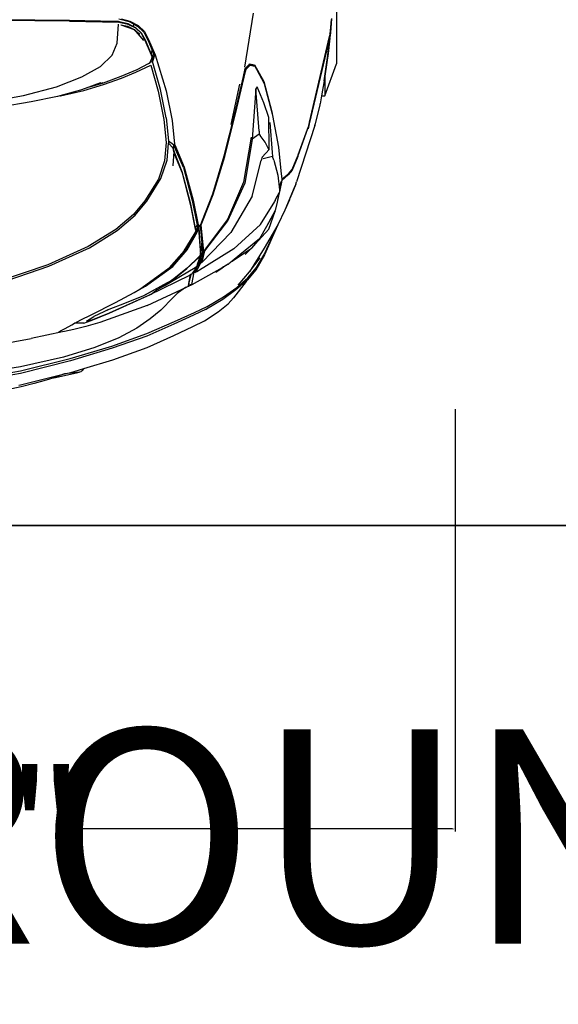
# Model space of a CAD drawing. Units: inches. Extents: x -4737294 to -4736756, y 1716389 to 1717040.
# Tile 5 of 25: x -4737133 to -4737096, y 1716424 to 1716491. Entities that reach past the tile are written whole.
import ezdxf

# ---------------------------------------------------------------- set-up
doc = ezdxf.new("R2010")
doc.units = ezdxf.units.IN
doc.header["$MEASUREMENT"] = 0
for name, color, linetype, lineweight in [('A-ANNO-DIMS', 2, 'Continuous', 18), ('A-ANNO-TEXT', 250, 'Continuous', 30), ('A-EQPM-VEHI', 250, 'Continuous', 13), ('walls', 252, 'Continuous', 35)]:
    doc.layers.add(name, color=color, linetype=linetype, lineweight=lineweight)
doc.layers.add('Edges', color=250, linetype='Continuous')
doc.styles.get("Standard").update_dxf_attribs({"font": 'arial.ttf'})
doc.dimstyles.get("Standard").update_dxf_attribs({"dimtxt": 8, "dimasz": 0.18, "dimexe": 0.18, "dimexo": 0.0625, "dimgap": 0.09, "dimtad": 0, "dimtih": 1, "dimtoh": 1, "dimzin": 0, "dimdsep": 46, "dimlunit": 3, "dimtxsty": 'Standard', "dimcen": 0.09, "dimadec": 0, "dimazin": 0, "dimtfac": 1, "dimtofl": 0, "dimtmove": 0, "dimatfit": 3, "dimfxl": 1, "dimtolj": 1, "dimtzin": 0, "dimarcsym": 0})

# ---------------------------------------------------------------- blocks, each defined once
blk = doc.blocks.new('Nissan Qashqai pl')
at = {"layer": 'Edges'}
for p, q in [((10.9577, 12.8101), (11.1283, 12.8101)), ((11.0576, 12.8026), (11.0798, 12.8008)), ((11.0768, 12.8008), (11.059, 12.8023)), ((11.0811, 12.8004), (11.0768, 12.8008)), ((11.0798, 12.8008), (11.0872, 12.7999)), ((11.0827, 12.8001), (11.0811, 12.8004)), ((11.0827, 12.8001), (11.0813, 12.7998)), ((11.0836, 12.8002), (11.0827, 12.8001)), ((11.0856, 12.7994), (11.0827, 12.8001)), ((11.0872, 12.7999), (11.0836, 12.8002)), ((11.0836, 12.8002), (11.0882, 12.7992)), ((11.2196, 12.7681), (11.0856, 12.7994)), ((11.0883, 12.7998), (11.0872, 12.7999)), ((11.0882, 12.7992), (11.2222, 12.7676)), ((11.0883, 12.7998), (11.1123, 12.797)), ((11.1147, 12.7965), (11.0883, 12.7998)), ((11.1123, 12.797), (11.1475, 12.7921)), ((11.1547, 12.791), (11.1147, 12.7965)), ((11.1783, 12.7921), (11.1283, 12.8101)), ((11.1475, 12.7921), (11.1525, 12.7914)), ((11.1475, 12.7921), (11.1783, 12.7921)), ((11.1525, 12.7914), (11.1547, 12.791)), ((11.1547, 12.791), (11.1783, 12.787)), ((11.1783, 12.787), (11.1783, 12.7921)), ((11.1783, 12.787), (11.1906, 12.7849)), ((11.1906, 12.7849), (11.1909, 12.7849)), ((11.193, 12.7845), (11.1909, 12.7849)), ((11.2215, 12.7775), (11.193, 12.7845)), ((11.2247, 12.767), (11.2163, 12.7689)), ((11.22, 12.768), (11.2196, 12.7681)), ((11.2247, 12.767), (11.22, 12.768)), ((11.2247, 12.7764), (11.2215, 12.7775)), ((11.2222, 12.7676), (11.2271, 12.7664)), ((11.2247, 12.7764), (11.3124, 12.7479)), ((11.2253, 12.7668), (11.2247, 12.767)), ((11.2304, 12.7649), (11.2253, 12.7668)), ((11.2253, 12.7668), (11.2271, 12.7664)), ((11.2271, 12.7664), (11.2296, 12.7658)), ((11.2271, 12.7664), (11.2277, 12.7662)), ((11.2277, 12.7662), (11.2296, 12.7658)), ((11.2732, 12.7496), (11.2277, 12.7662)), ((11.2704, 12.7504), (11.2304, 12.7649)), ((11.2702, 12.7507), (11.2704, 12.7504)), ((11.2704, 12.7506), (11.2707, 12.7503)), ((11.2707, 12.7503), (11.2704, 12.7504)), ((11.2719, 12.7498), (11.2707, 12.7503)), ((11.2934, 12.741), (11.2719, 12.7498)), ((11.2732, 12.7496), (11.2946, 12.7409)), ((11.3, 12.735), (11.2934, 12.741)), ((11.2946, 12.7409), (11.3018, 12.7346)), ((11.3081, 12.7253), (11.3, 12.735)), ((11.3018, 12.7346), (11.3103, 12.7249)), ((11.3161, 12.7467), (11.3124, 12.7479)), ((11.3161, 12.7467), (11.3376, 12.7381)), ((11.3192, 12.7454), (11.3566, 12.7294)), ((11.3405, 12.7369), (11.3376, 12.7381)), ((11.3405, 12.7369), (11.3566, 12.7294)), ((11.2091, 12.7103), (11.2583, 12.7196)), ((11.2583, 12.7196), (11.2956, 12.7234)), ((11.2956, 12.7234), (11.3085, 12.7247)), ((11.3022, 12.7186), (11.3252, 12.7213)), ((11.3086, 12.7247), (11.3081, 12.7253)), ((11.3081, 12.7253), (11.3087, 12.7247)), ((11.3085, 12.7247), (11.3086, 12.7247)), ((11.3086, 12.7247), (11.3087, 12.7247)), ((11.3087, 12.7247), (11.3103, 12.7249)), ((11.3103, 12.7249), (11.3103, 12.7249)), ((11.3103, 12.7249), (11.3106, 12.7249)), ((11.3106, 12.7249), (11.314, 12.7238)), ((11.317, 12.7227), (11.3119, 12.7236)), ((11.3132, 12.7243), (11.3256, 12.7215)), ((11.314, 12.7238), (11.317, 12.7227)), ((11.314, 12.7238), (11.3242, 12.7216)), ((11.3242, 12.7216), (11.317, 12.7227)), ((11.3198, 12.7211), (11.3252, 12.7213)), ((11.3242, 12.7216), (11.3256, 12.7215)), ((11.3252, 12.7213), (11.3283, 12.7214)), ((11.3256, 12.7215), (11.3283, 12.7214)), ((11.3283, 12.7214), (11.3297, 12.7206)), ((11.3297, 12.7206), (11.3446, 12.7173)), ((11.3297, 12.7206), (11.3302, 12.7203)), ((11.3302, 12.7203), (11.3446, 12.7173)), ((11.3302, 12.7203), (11.3394, 12.7152)), ((11.3566, 12.7294), (11.3796, 12.7187)), ((11.3796, 12.7187), (11.4164, 12.6974)), ((11.3796, 12.7187), (11.3807, 12.7182)), ((11.156, 12.6966), (11.203, 12.7093)), ((11.1589, 12.6971), (11.2062, 12.7098)), ((11.2121, 12.7043), (11.189, 12.6968)), ((11.203, 12.7093), (11.2091, 12.7103)), ((11.2062, 12.7098), (11.2091, 12.7103)), ((11.2622, 12.7051), (11.2121, 12.7043)), ((11.2199, 12.706), (11.2666, 12.7097)), ((11.2601, 12.7037), (11.2505, 12.6987)), ((11.2622, 12.7051), (11.2601, 12.7037)), ((11.2743, 12.6942), (11.2622, 12.7051)), ((11.2666, 12.7097), (11.2729, 12.7104)), ((11.2787, 12.7123), (11.2729, 12.7104)), ((11.2729, 12.7104), (11.2766, 12.6957)), ((11.2787, 12.7123), (11.3022, 12.7186)), ((11.3394, 12.7152), (11.3434, 12.7138)), ((11.3394, 12.7152), (11.342, 12.7137)), ((11.379, 12.6915), (11.3434, 12.7138)), ((11.3446, 12.7173), (11.3571, 12.7146)), ((11.3583, 12.7142), (11.3571, 12.7146)), ((11.3571, 12.7146), (11.3821, 12.7008)), ((11.3583, 12.7142), (11.3821, 12.7008)), ((11.3864, 12.7044), (11.3583, 12.7142)), ((11.3807, 12.7182), (11.4267, 12.6979)), ((11.4228, 12.6989), (11.3807, 12.7182)), ((11.4163, 12.6775), (11.3864, 12.7044)), ((11.1298, 12.6823), (11.156, 12.6966)), ((11.1365, 12.6851), (11.1589, 12.6971)), ((11.189, 12.6968), (11.1644, 12.6862)), ((11.2337, 12.6892), (11.1672, 12.6844)), ((11.2337, 12.6892), (11.2382, 12.6892)), ((11.2382, 12.6892), (11.2401, 12.6908)), ((11.2382, 12.6892), (11.2459, 12.6785)), ((11.2505, 12.6987), (11.2401, 12.6908)), ((11.2743, 12.6942), (11.2791, 12.6927)), ((11.335, 12.6786), (11.2791, 12.6927)), ((11.379, 12.6915), (11.417, 12.6499)), ((11.3821, 12.7008), (11.4014, 12.69)), ((11.4014, 12.69), (11.4022, 12.6894)), ((11.4014, 12.69), (11.4265, 12.6594)), ((11.4022, 12.6894), (11.4163, 12.6775)), ((11.4022, 12.6894), (11.4265, 12.6594)), ((11.4164, 12.6974), (11.4531, 12.6744)), ((11.4243, 12.6982), (11.4228, 12.6989)), ((11.4464, 12.6853), (11.4243, 12.6982)), ((11.4267, 12.6979), (11.4498, 12.6844)), ((11.4531, 12.6744), (11.4314, 12.6911)), ((11.1336, 12.667), (11.0492, 12.6807)), ((11.1285, 12.6745), (11.1298, 12.6823)), ((11.1293, 12.6736), (11.1285, 12.6745)), ((11.1306, 12.6812), (11.1293, 12.6736)), ((11.1353, 12.6677), (11.1293, 12.6736)), ((11.1306, 12.6752), (11.1319, 12.6827)), ((11.1319, 12.6827), (11.1306, 12.6812)), ((11.1347, 12.671), (11.1306, 12.6752)), ((11.1319, 12.6827), (11.1365, 12.6851)), ((11.1644, 12.6862), (11.1672, 12.6844)), ((11.1672, 12.6844), (11.2459, 12.6785)), ((11.2428, 12.6769), (11.3132, 12.6652)), ((11.2459, 12.6785), (11.3153, 12.6672)), ((11.335, 12.6786), (11.3915, 12.6453)), ((11.4366, 12.6471), (11.4163, 12.6775)), ((11.4163, 12.6775), (11.4259, 12.6674)), ((11.4624, 12.6717), (11.4464, 12.6853)), ((11.4498, 12.6844), (11.4662, 12.6706)), ((11.4681, 12.6691), (11.4498, 12.6844)), ((11.4742, 12.6567), (11.4531, 12.6744)), ((11.1366, 12.6691), (11.1347, 12.671)), ((11.1358, 12.6676), (11.1353, 12.6677)), ((11.1358, 12.6676), (11.1366, 12.6691)), ((11.148, 12.665), (11.1358, 12.6676)), ((11.1401, 12.6682), (11.1366, 12.6691)), ((11.2066, 12.6527), (11.1401, 12.6682)), ((11.2063, 12.6515), (11.148, 12.665)), ((11.2232, 12.6458), (11.1598, 12.6594)), ((11.3132, 12.6652), (11.3715, 12.6398)), ((11.3733, 12.6404), (11.3153, 12.6672)), ((11.4265, 12.6594), (11.4366, 12.6471)), ((11.4774, 12.6543), (11.4624, 12.6717)), ((11.4662, 12.6706), (11.4815, 12.6531)), ((11.4681, 12.6691), (11.4936, 12.6491)), ((11.272, 12.6349), (11.2063, 12.6515)), ((11.2728, 12.6357), (11.2066, 12.6527)), ((11.3915, 12.6453), (11.4381, 12.6002)), ((11.417, 12.6499), (11.4529, 12.5922)), ((11.4366, 12.6471), (11.4408, 12.6419)), ((11.4408, 12.6419), (11.4411, 12.6414)), ((11.4924, 12.6339), (11.4774, 12.6543)), ((11.4815, 12.6531), (11.4963, 12.6328)), ((11.4936, 12.6491), (11.5033, 12.6408)), ((11.3311, 12.6172), (11.272, 12.6349)), ((11.3323, 12.6178), (11.2728, 12.6357)), ((11.3715, 12.6398), (11.4177, 12.6052)), ((11.4203, 12.6044), (11.3733, 12.6404)), ((11.4411, 12.6414), (11.4411, 12.6414)), ((11.4414, 12.6409), (11.4411, 12.6414)), ((11.4414, 12.6409), (11.447, 12.6315)), ((11.4455, 12.6336), (11.4414, 12.6409)), ((11.447, 12.6315), (11.4455, 12.6336)), ((11.4455, 12.6336), (11.4462, 12.6324)), ((11.447, 12.6315), (11.4462, 12.6324)), ((11.4732, 12.585), (11.4462, 12.6324)), ((11.447, 12.6315), (11.447, 12.6314)), ((11.4536, 12.6215), (11.447, 12.6314)), ((11.5074, 12.608), (11.4924, 12.6339)), ((11.4964, 12.6326), (11.4963, 12.6328)), ((11.4964, 12.6326), (11.5113, 12.6069)), ((11.5158, 12.6256), (11.5033, 12.6408)), ((11.3751, 12.5999), (11.3311, 12.6172)), ((11.3747, 12.6011), (11.3323, 12.6178)), ((11.5295, 12.6041), (11.5158, 12.6256)), ((11.38, 12.5988), (11.3747, 12.6011)), ((11.3751, 12.5999), (11.3762, 12.5999)), ((11.3752, 12.5998), (11.3751, 12.5999)), ((11.3763, 12.5998), (11.3752, 12.5998)), ((11.3764, 12.5993), (11.3752, 12.5998)), ((11.3792, 12.5982), (11.3764, 12.5993)), ((11.3792, 12.5982), (11.3793, 12.5979)), ((11.3792, 12.5982), (11.3804, 12.5972)), ((11.3853, 12.5993), (11.38, 12.5988)), ((11.3804, 12.5972), (11.4082, 12.5998)), ((11.3827, 12.5953), (11.3804, 12.5972)), ((11.3811, 12.5958), (11.3808, 12.5961)), ((11.3846, 12.5953), (11.4248, 12.5976)), ((11.4212, 12.603), (11.3853, 12.5993)), ((11.3915, 12.5951), (11.4266, 12.5977)), ((11.409, 12.5999), (11.4082, 12.5998)), ((11.4164, 12.5998), (11.4082, 12.5998)), ((11.4152, 12.6004), (11.409, 12.5999)), ((11.409, 12.5999), (11.4163, 12.5999)), ((11.4173, 12.6006), (11.4152, 12.6004)), ((11.4163, 12.5999), (11.4152, 12.6004)), ((11.4163, 12.5999), (11.4186, 12.5999)), ((11.4164, 12.5998), (11.4163, 12.5999)), ((11.4181, 12.5998), (11.4164, 12.5998)), ((11.4169, 12.5996), (11.4164, 12.5998)), ((11.4252, 12.598), (11.4169, 12.5996)), ((11.4176, 12.6007), (11.4173, 12.6006)), ((11.418, 12.6006), (11.4173, 12.6006)), ((11.4215, 12.601), (11.4176, 12.6007)), ((11.418, 12.6006), (11.4176, 12.6007)), ((11.4177, 12.6052), (11.4193, 12.6042)), ((11.4204, 12.6002), (11.418, 12.6006)), ((11.4194, 12.6), (11.418, 12.6006)), ((11.4192, 12.6045), (11.4194, 12.6042)), ((11.4194, 12.6042), (11.4193, 12.6042)), ((11.4193, 12.6042), (11.4196, 12.604)), ((11.4194, 12.6042), (11.4196, 12.604)), ((11.4196, 12.6042), (11.4194, 12.6042)), ((11.4196, 12.604), (11.4201, 12.6036)), ((11.4198, 12.6041), (11.4201, 12.6036)), ((11.4201, 12.6036), (11.4212, 12.603)), ((11.4292, 12.6024), (11.4203, 12.6044)), ((11.4229, 12.6025), (11.4203, 12.6044)), ((11.4212, 12.603), (11.4215, 12.601)), ((11.4218, 12.6028), (11.4212, 12.603)), ((11.4215, 12.601), (11.4219, 12.6009)), ((11.4222, 12.6029), (11.4218, 12.6028)), ((11.4229, 12.6025), (11.4218, 12.6028)), ((11.4219, 12.6009), (11.4222, 12.6005)), ((11.4219, 12.6009), (11.4224, 12.6008)), ((11.4224, 12.6008), (11.4226, 12.6006)), ((11.4224, 12.6008), (11.423, 12.6006)), ((11.4315, 12.6002), (11.4229, 12.6025)), ((11.423, 12.6006), (11.4229, 12.6025)), ((11.44, 12.5959), (11.423, 12.6006)), ((11.4248, 12.5976), (11.4266, 12.5977)), ((11.4266, 12.5977), (11.4252, 12.598)), ((11.4266, 12.5977), (11.4268, 12.5977)), ((11.4268, 12.5977), (11.4296, 12.5954)), ((11.4268, 12.5977), (11.4278, 12.5977)), ((11.4303, 12.5956), (11.4278, 12.5977)), ((11.4278, 12.5977), (11.43, 12.5969)), ((11.4381, 12.6002), (11.4292, 12.6024)), ((11.4337, 12.5962), (11.43, 12.5969)), ((11.43, 12.5969), (11.4361, 12.5948)), ((11.4403, 12.5978), (11.4315, 12.6002)), ((11.4397, 12.5937), (11.4337, 12.5962)), ((11.4381, 12.6002), (11.4403, 12.5978)), ((11.4403, 12.5978), (11.44, 12.5959)), ((11.44, 12.5959), (11.4457, 12.5928)), ((11.4462, 12.5947), (11.4403, 12.5978)), ((11.5165, 12.5882), (11.5074, 12.608)), ((11.5113, 12.6068), (11.5113, 12.6069)), ((11.5113, 12.6068), (11.5206, 12.5869)), ((11.5384, 12.5859), (11.5295, 12.6041)), ((11.2895, 12.5724), (11.3411, 12.5863)), ((11.29, 12.5711), (11.3419, 12.585)), ((11.3474, 12.5827), (11.2972, 12.5692)), ((11.3493, 12.5828), (11.2993, 12.5695)), ((11.3411, 12.5863), (11.3795, 12.5939)), ((11.3419, 12.585), (11.3804, 12.5926)), ((11.3847, 12.5899), (11.3474, 12.5827)), ((11.3474, 12.5827), (11.3474, 12.5827)), ((11.3863, 12.5898), (11.3493, 12.5828)), ((11.3795, 12.5939), (11.3834, 12.5947)), ((11.3804, 12.5926), (11.3841, 12.5933)), ((11.3847, 12.5899), (11.3804, 12.5926)), ((11.3834, 12.5947), (11.3827, 12.5953)), ((11.3846, 12.5953), (11.3829, 12.5952)), ((11.3829, 12.5952), (11.3849, 12.5951)), ((11.388, 12.591), (11.3829, 12.5952)), ((11.3834, 12.5947), (11.3841, 12.5933)), ((11.3846, 12.5953), (11.3846, 12.5953)), ((11.3851, 12.5951), (11.3846, 12.5953)), ((11.3846, 12.5953), (11.3849, 12.5951)), ((11.3847, 12.5899), (11.3848, 12.5899)), ((11.388, 12.591), (11.3848, 12.5899)), ((11.3849, 12.5951), (11.3851, 12.5951)), ((11.3882, 12.5923), (11.3849, 12.5951)), ((11.3851, 12.5951), (11.3867, 12.5949)), ((11.4171, 12.5766), (11.3851, 12.5951)), ((11.3895, 12.5912), (11.3863, 12.5898)), ((11.3867, 12.5949), (11.3915, 12.5951)), ((11.3914, 12.5926), (11.3867, 12.5949)), ((11.3886, 12.5919), (11.3872, 12.5927)), ((11.3882, 12.5923), (11.3886, 12.5919)), ((11.3886, 12.5919), (11.3895, 12.5912)), ((11.3892, 12.5916), (11.3886, 12.5919)), ((11.3923, 12.5894), (11.3895, 12.5912)), ((11.4187, 12.5768), (11.3914, 12.5926)), ((11.4203, 12.5724), (11.3923, 12.5894)), ((11.4296, 12.5954), (11.4469, 12.5773)), ((11.4479, 12.5766), (11.4303, 12.5956)), ((11.4361, 12.5948), (11.4406, 12.5932)), ((11.4406, 12.5932), (11.4397, 12.5937)), ((11.4406, 12.5932), (11.4442, 12.592)), ((11.4442, 12.592), (11.4497, 12.589)), ((11.4462, 12.5893), (11.4442, 12.592)), ((11.4457, 12.5928), (11.4512, 12.5893)), ((11.452, 12.591), (11.4462, 12.5947)), ((11.475, 12.5409), (11.4462, 12.5893)), ((11.4497, 12.589), (11.4498, 12.5889)), ((11.4535, 12.5876), (11.4498, 12.5889)), ((11.4498, 12.5889), (11.4549, 12.5855)), ((11.4512, 12.5893), (11.4535, 12.5876)), ((11.4539, 12.5897), (11.452, 12.591)), ((11.4529, 12.5922), (11.4542, 12.5894)), ((11.4535, 12.5876), (11.4532, 12.5882)), ((11.4535, 12.5876), (11.4542, 12.5894)), ((11.4535, 12.5876), (11.4728, 12.5838)), ((11.4542, 12.5894), (11.4539, 12.5897)), ((11.4549, 12.5855), (11.4568, 12.5836)), ((11.4564, 12.5833), (11.4567, 12.5833)), ((11.4569, 12.583), (11.4565, 12.5831)), ((11.4568, 12.5836), (11.4571, 12.5833)), ((11.4571, 12.5833), (11.4573, 12.583)), ((11.4573, 12.583), (11.4578, 12.5822)), ((11.4704, 12.5803), (11.4573, 12.583)), ((11.4573, 12.5823), (11.4574, 12.5822)), ((11.4573, 12.5823), (11.4573, 12.5823)), ((11.4576, 12.5822), (11.4574, 12.5822)), ((11.4578, 12.5822), (11.4588, 12.5807)), ((11.4605, 12.5816), (11.4578, 12.5822)), ((11.4588, 12.5807), (11.4895, 12.5178)), ((11.4713, 12.5794), (11.4605, 12.5816)), ((11.4742, 12.5797), (11.4704, 12.5803)), ((11.4732, 12.585), (11.4728, 12.5838)), ((11.4728, 12.5838), (11.4742, 12.5797)), ((11.4728, 12.5838), (11.4746, 12.5796)), ((11.4758, 12.5791), (11.4732, 12.585)), ((11.5306, 12.5573), (11.5165, 12.5882)), ((11.5206, 12.5869), (11.5349, 12.5559)), ((11.5527, 12.5559), (11.5384, 12.5859)), ((11.29, 12.5711), (11.2541, 12.5557)), ((11.2586, 12.5591), (11.2895, 12.5724)), ((11.2972, 12.5692), (11.2677, 12.5575)), ((11.2993, 12.5695), (11.2705, 12.5579)), ((11.4433, 12.5543), (11.4171, 12.5766)), ((11.4447, 12.5545), (11.4187, 12.5768)), ((11.4467, 12.5488), (11.4203, 12.5724)), ((11.4469, 12.5773), (11.4659, 12.5539)), ((11.4654, 12.5548), (11.4479, 12.5766)), ((11.4744, 12.5792), (11.4713, 12.5794)), ((11.4742, 12.5797), (11.4744, 12.5792)), ((11.4745, 12.5797), (11.4742, 12.5797)), ((11.4745, 12.5792), (11.4744, 12.5792)), ((11.4745, 12.5792), (11.4745, 12.5797)), ((11.4745, 12.5797), (11.4746, 12.5796)), ((11.4748, 12.5792), (11.4745, 12.5792)), ((11.4746, 12.5796), (11.4748, 12.5792)), ((11.4746, 12.5796), (11.4758, 12.5791)), ((11.4758, 12.5791), (11.4748, 12.5792)), ((11.4758, 12.5791), (11.4759, 12.579)), ((11.4759, 12.579), (11.4778, 12.5746)), ((11.4759, 12.579), (11.4771, 12.576)), ((11.5057, 12.5145), (11.4771, 12.576)), ((11.4778, 12.5746), (11.4826, 12.5669)), ((11.4826, 12.5669), (11.4869, 12.5615)), ((11.1702, 12.5444), (11.2166, 12.5534)), ((11.2166, 12.5534), (11.2538, 12.5571)), ((11.2488, 12.548), (11.2541, 12.5557)), ((11.2599, 12.5552), (11.2524, 12.5477)), ((11.2538, 12.5571), (11.2586, 12.5591)), ((11.2541, 12.5557), (11.2599, 12.5552)), ((11.2677, 12.5575), (11.2599, 12.5552)), ((11.265, 12.5563), (11.2599, 12.5552)), ((11.2705, 12.5579), (11.265, 12.5563)), ((11.265, 12.5563), (11.2724, 12.5557)), ((11.2724, 12.5557), (11.2874, 12.5544)), ((11.4745, 12.5116), (11.4433, 12.5543)), ((11.4758, 12.5118), (11.4447, 12.5545)), ((11.4633, 12.5594), (11.4897, 12.5108)), ((11.4654, 12.5548), (11.4659, 12.5539)), ((11.4659, 12.5539), (11.4674, 12.5512)), ((11.4675, 12.551), (11.4674, 12.5512)), ((11.4675, 12.551), (11.4703, 12.546)), ((11.4869, 12.5615), (11.4933, 12.555)), ((11.5131, 12.5356), (11.4933, 12.555)), ((11.5496, 12.5141), (11.5306, 12.5573)), ((11.5349, 12.5559), (11.5535, 12.5139)), ((11.5716, 12.5145), (11.5527, 12.5559)), ((11.1144, 12.5271), (11.1702, 12.5444)), ((11.1683, 12.5354), (11.1244, 12.5227)), ((11.2127, 12.5443), (11.1683, 12.5354)), ((11.1712, 12.5317), (11.2152, 12.5404)), ((11.2127, 12.5443), (11.2488, 12.548)), ((11.2152, 12.5404), (11.2509, 12.5439)), ((11.2488, 12.548), (11.2524, 12.5477)), ((11.2509, 12.5439), (11.28, 12.5414)), ((11.2785, 12.5455), (11.2524, 12.5477)), ((11.3076, 12.5358), (11.2785, 12.5455)), ((11.28, 12.5414), (11.3082, 12.532)), ((11.3428, 12.5139), (11.3076, 12.5358)), ((11.4801, 12.503), (11.4467, 12.5488)), ((11.4703, 12.546), (11.4704, 12.5458)), ((11.4704, 12.5458), (11.4909, 12.5085)), ((11.4704, 12.5458), (11.4897, 12.5108)), ((11.475, 12.5409), (11.4828, 12.5276)), ((11.5131, 12.5356), (11.5265, 12.5194)), ((11.0902, 12.5166), (11.1144, 12.5271)), ((11.0908, 12.5153), (11.107, 12.5224)), ((11.1138, 12.5213), (11.0912, 12.5117)), ((11.1149, 12.5212), (11.0917, 12.5114)), ((11.107, 12.5224), (11.1116, 12.5243)), ((11.1138, 12.5213), (11.107, 12.5224)), ((11.1116, 12.5243), (11.1147, 12.5257)), ((11.1244, 12.5227), (11.1116, 12.5243)), ((11.1139, 12.5213), (11.1138, 12.5213)), ((11.1164, 12.5224), (11.1139, 12.5213)), ((11.1147, 12.5257), (11.1244, 12.5227)), ((11.1172, 12.5222), (11.1149, 12.5212)), ((11.1164, 12.5224), (11.1174, 12.5223)), ((11.1173, 12.5222), (11.1172, 12.5222)), ((11.1174, 12.5223), (11.1173, 12.5222)), ((11.12, 12.5215), (11.1174, 12.5223)), ((11.1246, 12.5199), (11.12, 12.5215)), ((11.1259, 12.5194), (11.1244, 12.5227)), ((11.1244, 12.5227), (11.126, 12.5194)), ((11.1259, 12.5194), (11.1246, 12.5199)), ((11.126, 12.5193), (11.1247, 12.5197)), ((11.126, 12.5193), (11.1248, 12.5195)), ((11.1251, 12.5189), (11.126, 12.5193)), ((11.126, 12.5193), (11.1259, 12.5194)), ((11.126, 12.5194), (11.1259, 12.5194)), ((11.126, 12.5194), (11.1261, 12.5193)), ((11.1264, 12.5192), (11.126, 12.5194)), ((11.1263, 12.5186), (11.126, 12.5193)), ((11.1261, 12.5193), (11.126, 12.5193)), ((11.1261, 12.5193), (11.1263, 12.5188)), ((11.1264, 12.5192), (11.1261, 12.5193)), ((11.1277, 12.5167), (11.1264, 12.5192)), ((11.1302, 12.52), (11.1712, 12.5317)), ((11.1412, 12.4969), (11.1302, 12.52)), ((11.3082, 12.532), (11.3425, 12.5106)), ((11.488, 12.5208), (11.4828, 12.5276)), ((11.5179, 12.4551), (11.488, 12.5208)), ((11.5265, 12.5194), (11.541, 12.4982)), ((11.0682, 12.5004), (11.0779, 12.5103)), ((11.0692, 12.4996), (11.0787, 12.5092)), ((11.0802, 12.5057), (11.0718, 12.4967)), ((11.0809, 12.5056), (11.0727, 12.4966)), ((11.0747, 12.4944), (11.092, 12.5087)), ((11.0779, 12.5103), (11.0902, 12.5166)), ((11.0787, 12.5092), (11.0908, 12.5153)), ((11.0912, 12.5117), (11.0802, 12.5057)), ((11.0917, 12.5114), (11.0809, 12.5056)), ((11.1369, 12.4986), (11.1277, 12.5167)), ((11.3425, 12.5106), (11.3635, 12.4929)), ((11.3645, 12.4958), (11.3428, 12.5139)), ((11.4788, 12.5052), (11.4745, 12.5116)), ((11.4852, 12.494), (11.4758, 12.5118)), ((11.4801, 12.503), (11.4788, 12.5052)), ((11.4898, 12.5172), (11.4895, 12.5178)), ((11.4897, 12.5108), (11.4909, 12.5085)), ((11.4898, 12.5172), (11.49, 12.5167)), ((11.49, 12.5167), (11.5179, 12.4551)), ((11.4909, 12.5085), (11.5028, 12.4792)), ((11.5057, 12.5145), (11.5325, 12.4404)), ((11.5691, 12.4592), (11.5496, 12.5141)), ((11.5535, 12.5139), (11.5726, 12.46)), ((11.5908, 12.4606), (11.5716, 12.5145)), ((11.0614, 12.4872), (11.0682, 12.5004)), ((11.0624, 12.4866), (11.0658, 12.4932)), ((11.0658, 12.4932), (11.0692, 12.4996)), ((11.0658, 12.4932), (11.0698, 12.4925)), ((11.0698, 12.4925), (11.0659, 12.4848)), ((11.0727, 12.4966), (11.0669, 12.4849)), ((11.0671, 12.4731), (11.0747, 12.4944)), ((11.0696, 12.4836), (11.0747, 12.4944)), ((11.0718, 12.4967), (11.0698, 12.4925)), ((11.0747, 12.4944), (11.0821, 12.5029)), ((11.1475, 12.4741), (11.1369, 12.4986)), ((11.1505, 12.4742), (11.1412, 12.4969)), ((11.3635, 12.4929), (11.3872, 12.4654)), ((11.3888, 12.4678), (11.3645, 12.4958)), ((11.4852, 12.494), (11.4801, 12.503)), ((11.5013, 12.4651), (11.4852, 12.494)), ((11.541, 12.4982), (11.5562, 12.4701)), ((11.0581, 12.4738), (11.0614, 12.4872)), ((11.0582, 12.47), (11.0624, 12.4866)), ((11.063, 12.4728), (11.0622, 12.4697)), ((11.0659, 12.4848), (11.063, 12.4728)), ((11.0641, 12.4733), (11.0632, 12.47)), ((11.0669, 12.4849), (11.0641, 12.4733)), ((11.0671, 12.4731), (11.0696, 12.4836)), ((11.1577, 12.4465), (11.1475, 12.4741)), ((11.1605, 12.4465), (11.1505, 12.4742)), ((11.5028, 12.4792), (11.5118, 12.4548)), ((11.0621, 12.4657), (11.0607, 12.3933)), ((11.0618, 12.3933), (11.0632, 12.47)), ((11.0622, 12.4697), (11.0621, 12.4657)), ((11.0962, 12.4675), (11.0662, 12.4698)), ((11.1148, 12.4598), (11.0962, 12.4675)), ((11.1323, 12.4415), (11.1148, 12.4598)), ((11.3872, 12.4654), (11.4138, 12.4223)), ((11.4159, 12.4242), (11.3888, 12.4678)), ((11.5202, 12.427), (11.5013, 12.4651)), ((11.5562, 12.4701), (11.5715, 12.4326)), ((11.5884, 12.3943), (11.5691, 12.4592)), ((11.5726, 12.46), (11.5922, 12.3947)), ((11.6042, 12.4156), (11.5908, 12.4606)), ((11.1643, 12.425), (11.1576, 12.4459)), ((11.1643, 12.425), (11.1577, 12.4465)), ((11.1583, 12.4423), (11.1643, 12.425)), ((11.1699, 12.4153), (11.1605, 12.4465)), ((11.5118, 12.4548), (11.523, 12.4311)), ((11.5118, 12.4548), (11.513, 12.4514)), ((11.5292, 12.4272), (11.5179, 12.4551)), ((11.5179, 12.4551), (11.5285, 12.4279)), ((11.1487, 12.4126), (11.1323, 12.4415)), ((11.1582, 12.4416), (11.1668, 12.4177)), ((11.5283, 12.4109), (11.5202, 12.427)), ((11.5301, 12.4198), (11.523, 12.4311)), ((11.5285, 12.4279), (11.5302, 12.4209)), ((11.5331, 12.4157), (11.5292, 12.4272)), ((11.5325, 12.4404), (11.5386, 12.4187)), ((11.5715, 12.4326), (11.5866, 12.3835)), ((11.164, 12.373), (11.1487, 12.4126)), ((11.1643, 12.425), (11.1668, 12.4177)), ((11.1668, 12.4177), (11.1694, 12.4104)), ((11.178, 12.379), (11.1699, 12.4153)), ((11.4138, 12.4223), (11.4422, 12.3594)), ((11.4445, 12.3608), (11.4159, 12.4242)), ((11.5302, 12.4209), (11.5301, 12.4198)), ((11.5331, 12.4157), (11.5335, 12.401)), ((11.5386, 12.4187), (11.5434, 12.3997)), ((11.6042, 12.4156), (11.6077, 12.4125)), ((11.6103, 12.395), (11.6042, 12.4156)), ((11.6077, 12.4125), (11.6094, 12.4107)), ((11.1694, 12.4104), (11.1781, 12.3782)), ((11.5334, 12.4014), (11.5283, 12.4109)), ((11.5326, 12.4045), (11.5333, 12.4019)), ((11.5333, 12.4019), (11.5334, 12.4014)), ((11.5335, 12.401), (11.5334, 12.4014)), ((11.5357, 12.3968), (11.5335, 12.401)), ((11.5416, 12.3863), (11.5357, 12.3968)), ((11.5434, 12.3997), (11.5461, 12.3854)), ((11.6094, 12.4107), (11.6101, 12.4085)), ((11.6101, 12.4085), (11.6127, 12.3852)), ((11.6185, 12.3689), (11.6101, 12.4085)), ((11.0607, 12.3933), (11.0595, 12.2842)), ((11.0618, 12.3933), (11.0606, 12.2841)), ((11.5455, 12.3793), (11.5416, 12.3863)), ((11.5461, 12.3854), (11.5467, 12.3822)), ((11.5467, 12.3822), (11.5571, 12.3331)), ((11.5866, 12.3835), (11.6016, 12.3166)), ((11.6076, 12.3166), (11.5884, 12.3943)), ((11.5922, 12.3947), (11.6118, 12.3165)), ((11.6127, 12.3852), (11.6103, 12.395)), ((11.6127, 12.3852), (11.6174, 12.3722)), ((11.6297, 12.3166), (11.6127, 12.3852)), ((11.1776, 12.3211), (11.164, 12.373)), ((11.1781, 12.3782), (11.178, 12.379)), ((11.1781, 12.3782), (11.1791, 12.3746)), ((11.1791, 12.3746), (11.1877, 12.333)), ((11.5472, 12.3757), (11.5455, 12.3793)), ((11.6174, 12.3722), (11.6185, 12.3689)), ((11.6185, 12.3689), (11.6224, 12.3567)), ((11.4422, 12.3594), (11.4712, 12.2729)), ((11.4738, 12.274), (11.4445, 12.3608)), ((11.6224, 12.3567), (11.6277, 12.3379)), ((11.6277, 12.3379), (11.6328, 12.3174)), ((11.1891, 12.2586), (11.1776, 12.3211)), ((11.1877, 12.333), (11.1958, 12.2844)), ((11.5668, 12.2816), (11.5571, 12.3331)), ((11.6016, 12.3166), (11.615, 12.2333)), ((11.6229, 12.2274), (11.6076, 12.3166)), ((11.6118, 12.3165), (11.6272, 12.2272)), ((11.6301, 12.3141), (11.6297, 12.3166)), ((11.6328, 12.3174), (11.6375, 12.2956))]:
    blk.add_line(p, q, dxfattribs=at)
blk = doc.blocks.new('car')
blk.add_blockref('Nissan Qashqai pl', (-9.7433, -11.9151))
blk = doc.blocks.new('*D60')
at = {"layer": 'A-ANNO-DIMS', "color": 0, "lineweight": -2, "transparency": 16777216}
for p, q in [((-4737196.476, 1716464.781), (-4737196.476, 1716436.041)), ((-4737102.951, 1716464.781), (-4737102.951, 1716436.041)), ((-4737196.296, 1716436.221), (-4737169.725, 1716436.221)), ((-4737103.131, 1716436.221), (-4737129.703, 1716436.221))]:
    blk.add_line(p, q, dxfattribs=at)
at = {"layer": 'A-ANNO-DIMS', "color": 0, "transparency": 16777216}
for points in [[(-4737196.296, 1716436.251), (-4737196.296, 1716436.191), (-4737196.476, 1716436.221)], [(-4737103.131, 1716436.251), (-4737103.131, 1716436.191), (-4737102.951, 1716436.221)]]:
    blk.add_solid(points, dxfattribs=at)
at = {"layer": 'Defpoints', "color": 0, "transparency": 16777216}
for p in [(-4737196.476, 1716464.844), (-4737102.951, 1716464.844), (-4737102.951, 1716436.221)]:
    blk.add_point(p, dxfattribs=at)
at = {"layer": 'A-ANNO-DIMS', "color": 0, "transparency": 16777216, "insert": (-4737149.714, 1716436.221), "char_height": 8, "attachment_point": 5}
blk.add_mtext('\\A1;7\'-9 1/2"', dxfattribs=at)

msp = doc.modelspace()

# ---------------------------------------------------------------- linework, layer by layer
at = {"layer": 'walls'}
msp.add_line((-4737215.144, 1716456.869), (-4737062.144, 1716456.869), dxfattribs=at)

# ---------------------------------------------------------------- block references
at = {"layer": 'A-EQPM-VEHI', "xscale": 43.56002006885659, "yscale": 43.56002006885659, "zscale": 43.56002006885659, "rotation": 270}
msp.add_blockref('car', (-4737150.017, 1716548.61), dxfattribs=at)

# ---------------------------------------------------------------- texts
at = {"layer": 'A-ANNO-TEXT'}
msp.add_text('GROUND FLOOR PLAN', height=14.58777, dxfattribs=at).set_placement((-4737157.681, 1716428.409))

# ---------------------------------------------------------------- dimensions: what is measured, and where the dimension line sits
at = {"layer": 'A-ANNO-DIMS'}
dim = msp.add_linear_dim(base=(-4737102.951, 1716436.221), p1=(-4737196.476, 1716464.844), p2=(-4737102.951, 1716464.844), dimstyle='Standard', override={"dimdec": 1, "dimlfac": 1, "dimrnd": 0, "dimzin": 1, "dimdsep": 46, "dimlunit": 4, "dimfrac": 2}, dxfattribs=at)
dim.commit()
dim.dimension.update_dxf_attribs({"geometry": '*D60', "text_midpoint": (-4737149.714, 1716436.221)})

doc.saveas('drawing.dxf')
